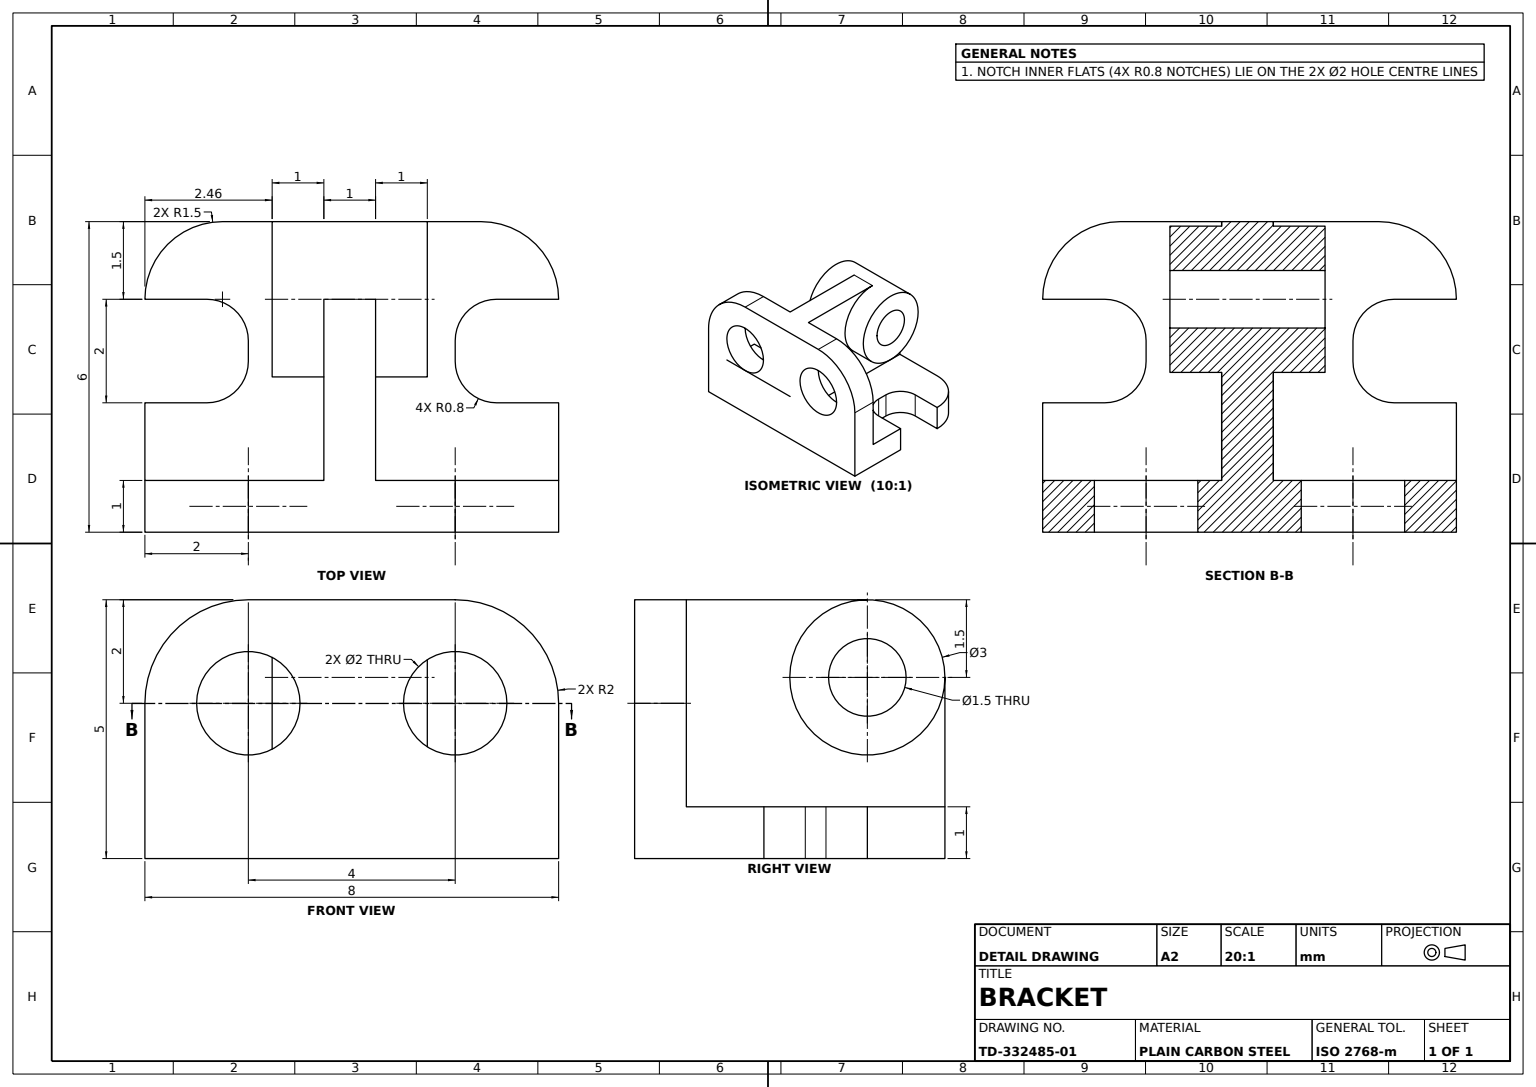
from build123d import *

# Parameters (mm, degrees)
BASE_PLATE_DEPTH       = 1
UPRIGHT_PLATE_SKETCH_R = 1
UPRIGHT_PLATE_DEPTH    = 1
RIB_SKETCH_W           = 1
RIB_SKETCH_H           = 4
RIB_DEPTH              = 5
PIVOT_HUB_DEPTH        = 1
PIVOT_HUB_DEPTH_BACK   = 2
PIVOT_HUB_SKETCH_R     = 1.5
HUB_BORE_SKETCH_R      = 0.75
HUB_BORE_DEPTH         = 3
SLOT_CUT_DEPTH         = 3


with BuildPart() as part:
    # Base Plate Sketch → Base Plate (new body)
    with BuildSketch(Plane(origin=(0, 0, 0), x_dir=(1, 0, 0), z_dir=(0, 1, 0))):
        with BuildLine():
            Line((-4, 1.5), (-2.8, 1.5))
            ThreePointArc((-2.8, 1.5), (-2.234314575, 1.265685425), (-2, 0.7))
            Line((-2, 0.7), (-2, 0.3))
            ThreePointArc((-2, 0.3), (-2.234314575, -0.265685425), (-2.8, -0.5))
            Line((-2.8, -0.5), (-4, -0.5))
            Line((-4, -0.5), (-4, -3))
            Line((-4, -3), (4, -3))
            Line((4, -3), (4, -0.5))
            Line((4, -0.5), (2.8, -0.5))
            ThreePointArc((2.8, -0.5), (2.234314575, -0.265685425), (2, 0.3))
            Line((2, 0.3), (2, 0.7))
            ThreePointArc((2, 0.7), (2.234314575, 1.265685425), (2.8, 1.5))
            Line((2.8, 1.5), (4, 1.5))
            ThreePointArc((4, 1.5), (3.560660172, 2.560660172), (2.5, 3))
            Line((2.5, 3), (-2.5, 3))
            ThreePointArc((-2.5, 3), (-3.560660172, 2.560660172), (-4, 1.5))
        make_face()
    extrude(amount=BASE_PLATE_DEPTH)

    # Upright Plate Sketch → Upright Plate (add)
    with BuildSketch(Plane.XY.offset(3)):
        with BuildLine():
            Line((-4, 0), (4, 0))
            Line((4, 0), (4, 3))
            ThreePointArc((4, 3), (3.414213562, 4.414213562), (2, 5))
            Line((2, 5), (-2, 5))
            ThreePointArc((-2, 5), (-3.414213562, 4.414213562), (-4, 3))
            Line((-4, 3), (-4, 0))
        make_face()
        with Locations((-2, 3)):
            Circle(UPRIGHT_PLATE_SKETCH_R, mode=Mode.SUBTRACT)
        with Locations((2, 3)):
            Circle(UPRIGHT_PLATE_SKETCH_R, mode=Mode.SUBTRACT)
    extrude(amount=-UPRIGHT_PLATE_DEPTH)

    # Rib Sketch → Rib (add)
    with BuildSketch(Plane(origin=(0, 0, 2), x_dir=(-1, 0, 0), z_dir=(0, 0, -1))):
        with Locations((0.039501807, 3)):
            Rectangle(RIB_SKETCH_W, RIB_SKETCH_H)
    extrude(amount=RIB_DEPTH)

    # Pivot Hub Sketch → Pivot Hub (add, two sides: drawn at the far end of the back side and taken through both)
    with BuildSketch(Plane(origin=(0.460498193, 0, 0), x_dir=(0, 0, -1), z_dir=(1, 0, 0)).offset(-PIVOT_HUB_DEPTH_BACK)):
        with Locations((1.5, 3.5)):
            Circle(PIVOT_HUB_SKETCH_R)
    extrude(amount=PIVOT_HUB_DEPTH + PIVOT_HUB_DEPTH_BACK)

    # Hub Bore Sketch → Hub Bore (cut)
    with BuildSketch(Plane(origin=(1.460498193, 0, 0), x_dir=(0, 0, -1), z_dir=(1, 0, 0))):
        with Locations((1.5, 3.5)):
            Circle(HUB_BORE_SKETCH_R)
    extrude(amount=-HUB_BORE_DEPTH, mode=Mode.SUBTRACT)

    # Slot Cut Sketch → Slot Cut (cut)
    with BuildSketch(Plane(origin=(0.460498193, 0, 0), x_dir=(0, 0, -1), z_dir=(1, 0, 0))):
        with BuildLine():
            Line((1.5, 5), (3, 5))
            Line((3, 5), (3, 3.5))
            ThreePointArc((3, 3.5), (2.560660172, 4.560660172), (1.5, 5))
        make_face()
    extrude(amount=-SLOT_CUT_DEPTH, mode=Mode.SUBTRACT)


solid = part.part
